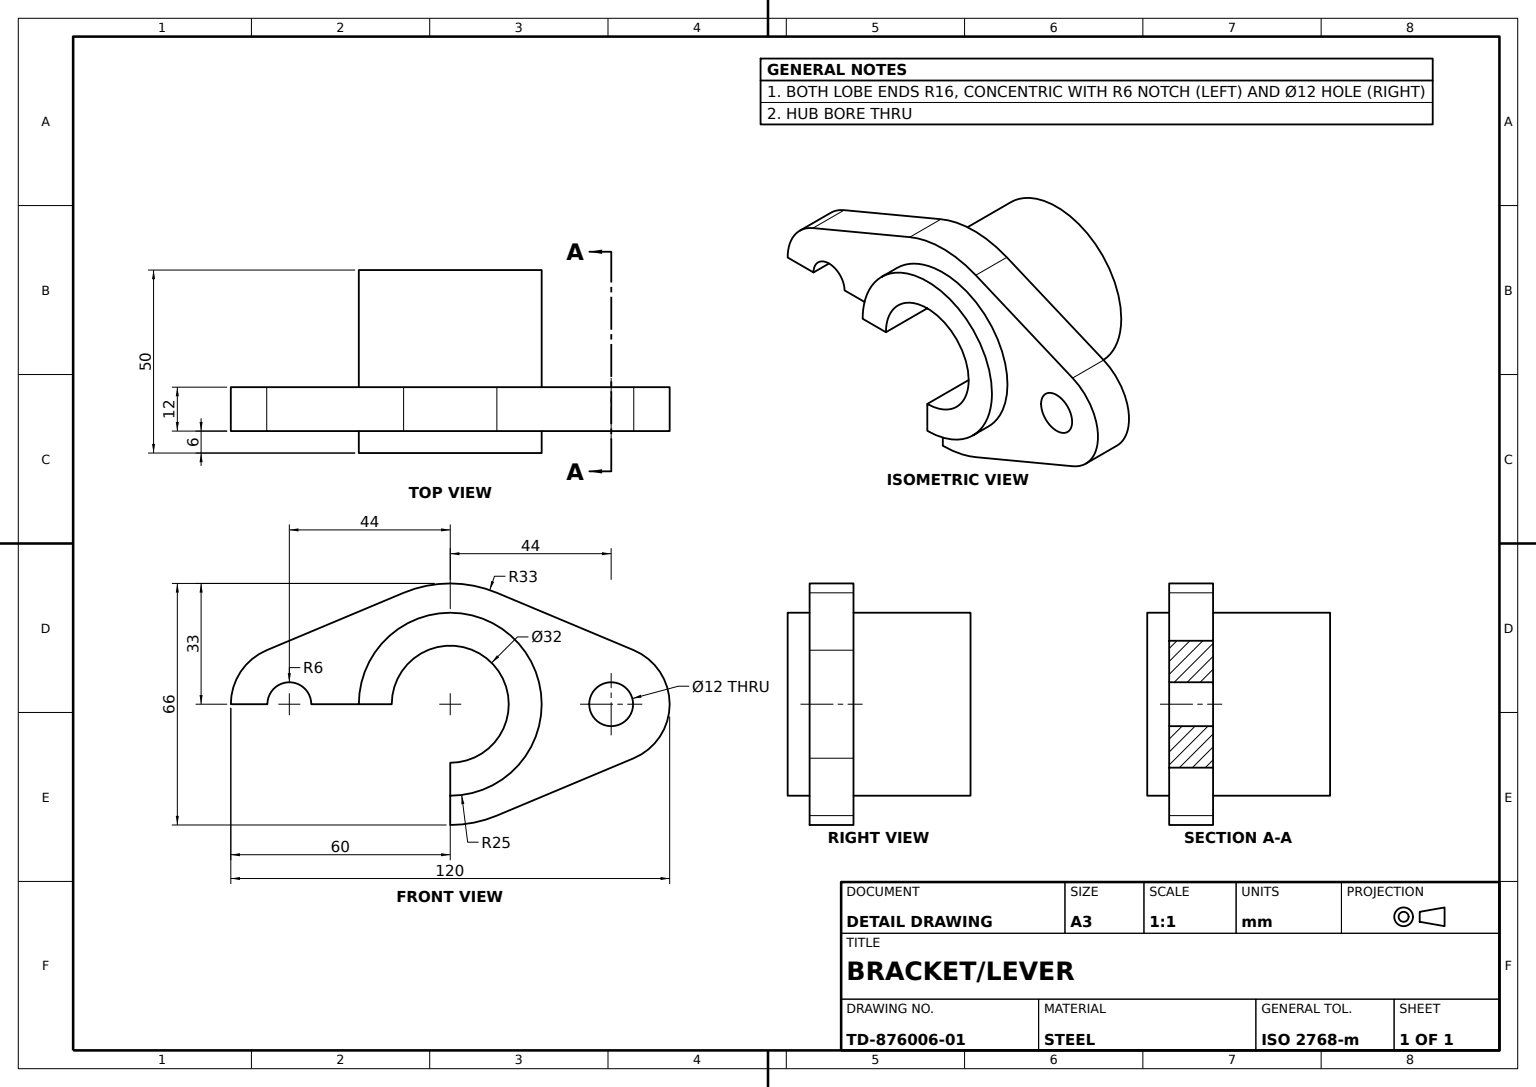
from build123d import *

# Parameters (mm, degrees)
BRACKET_PLATE_PROFILE_R  = 6
BRACKET_PLATE_12MM_DEPTH = 6
HUB_AND_BORE_CIRCLES_R   = 16
BORE_32_DEPTH            = 12
HUB_50_DEPTH             = 6
HUB_50_DEPTH_BACK        = 44
SKETCH2_3_R              = 25
SKETCH2_3_R_2            = 16
HUB_SLOT_CUT_DEPTH       = 85.787970845


with BuildPart() as part:
    # Bracket Plate Profile → Bracket Plate 12mm (new, symmetric)
    with BuildSketch(Plane.XY):
        with BuildLine():
            Line((12.75, 30.437435832), (50.181818182, 14.757544646))
            ThreePointArc((50.181818182, 14.757544646), (60, 0), (50.181818182, -14.757544646))
            Line((50.181818182, -14.757544646), (12.75, -30.437435832))
            ThreePointArc((12.75, -30.437435832), (0, -33), (-12.75, -30.437435832))
            Line((-12.75, -30.437435832), (-50.181818182, -14.757544646))
            ThreePointArc((-50.181818182, -14.757544646), (-60, 0), (-50.181818182, 14.757544646))
            Line((-50.181818182, 14.757544646), (-12.75, 30.437435832))
            ThreePointArc((-12.75, 30.437435832), (0, 33), (12.75, 30.437435832))
        make_face()
        with Locations((-44, 0)):
            Circle(BRACKET_PLATE_PROFILE_R, mode=Mode.SUBTRACT)
        with Locations((44, 0)):
            Circle(BRACKET_PLATE_PROFILE_R, mode=Mode.SUBTRACT)
    extrude(amount=BRACKET_PLATE_12MM_DEPTH, both=True)

    # Hub and Bore Circles → Bore _32 (cut)
    with BuildSketch(Plane.XY.offset(6)):
        Circle(HUB_AND_BORE_CIRCLES_R)
    extrude(amount=-BORE_32_DEPTH, mode=Mode.SUBTRACT)

    # Sketch2_3 → Hub _50 (add, two sides: drawn at the far end of the back side and taken through both)
    with BuildSketch(Plane.XY.offset(6).offset(-HUB_50_DEPTH_BACK)):
        Circle(SKETCH2_3_R)
        Circle(SKETCH2_3_R_2, mode=Mode.SUBTRACT)
    extrude(amount=HUB_50_DEPTH + HUB_50_DEPTH_BACK)

    # Hub Slot Profile → Hub Slot Cut (cut, through all)
    with BuildSketch(Plane(origin=(0, 0, -38), x_dir=(-1, 0, 0), z_dir=(0, 0, -1))):
        Polygon((0, 0), (0, -33), (0, -48.621178417), (74.791991636, 0), (30.829460929, 0), align=None)
    extrude(amount=-HUB_SLOT_CUT_DEPTH, mode=Mode.SUBTRACT)


solid = part.part
